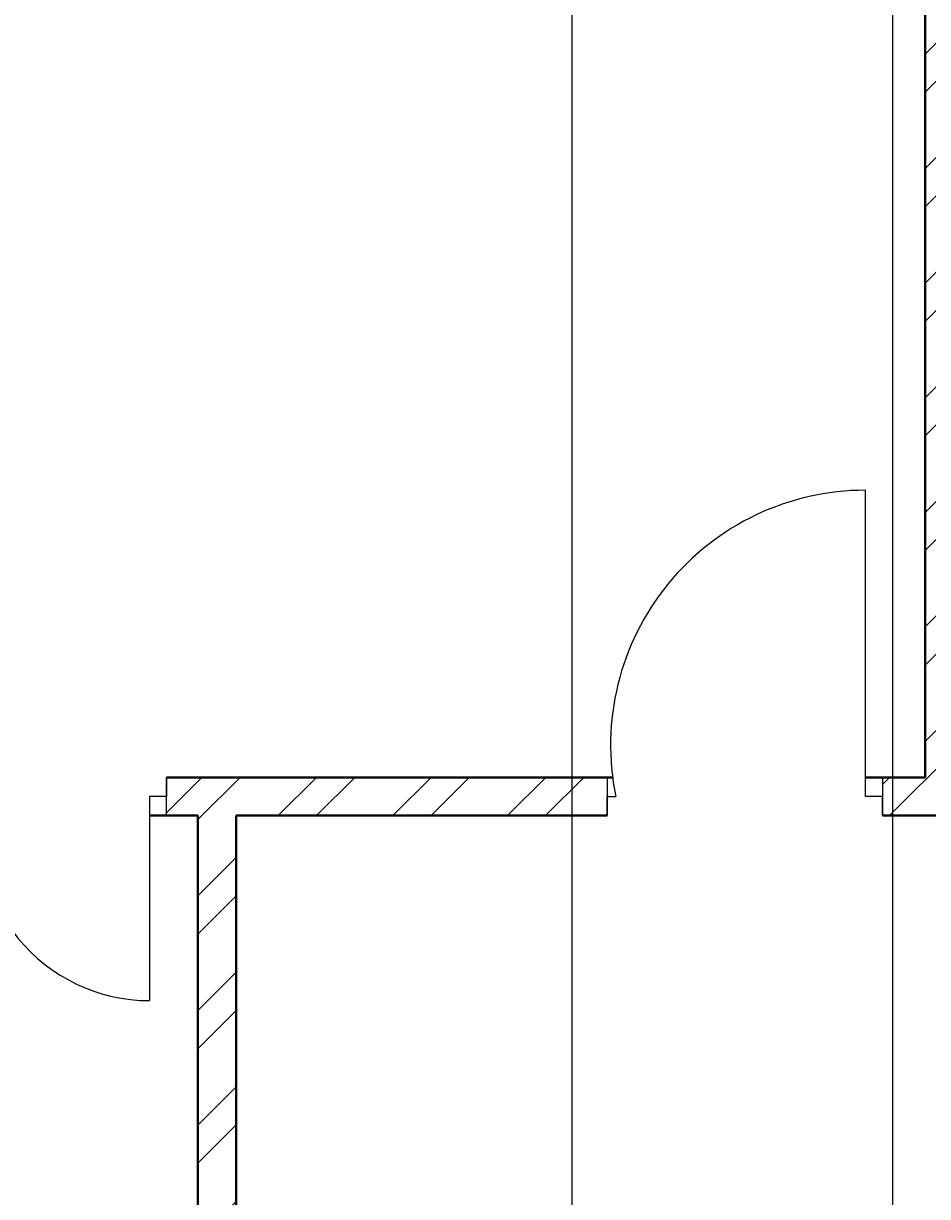
# Model space of a CAD drawing. Units: inches. Extents: x 1601 to 2297, y 1496 to 2631.
# Tile 8 of 57: x 1783 to 1889, y 1835 to 1973. Entities that reach past the tile are written whole.
import ezdxf

# ---------------------------------------------------------------- set-up
doc = ezdxf.new("R2010")
doc.units = ezdxf.units.IN
for name, color, linetype, lineweight in [('A-ANNO-DIMS', 2, 'Continuous', 18), ('A-DOOR', 21, 'Continuous', 25), ('A-WALL', 7, 'Continuous', 40), ('A-WALL-PATT', 215, 'Continuous', 13)]:
    doc.layers.add(name, color=color, linetype=linetype, lineweight=lineweight)
doc.styles.get("Standard").update_dxf_attribs({"font": 'arial.ttf'})
doc.dimstyles.get("Standard").update_dxf_attribs({"dimtxt": 0.18, "dimasz": 0.18, "dimexe": 0.18, "dimexo": 0.0625, "dimgap": 0.09, "dimtad": 0, "dimtih": 1, "dimtoh": 1, "dimdec": 4, "dimzin": 0, "dimdsep": 46, "dimtxsty": 'Standard', "dimcen": 0.09, "dimadec": 0, "dimazin": 0, "dimtfac": 1, "dimtdec": 4, "dimtofl": 0, "dimtmove": 0, "dimatfit": 3, "dimfxl": 1, "dimtolj": 1, "dimtzin": 0, "dimarcsym": 0})

# ---------------------------------------------------------------- blocks, each defined once
blk = doc.blocks.new('*D46')
at = {"layer": 'A-ANNO-DIMS', "color": 0, "lineweight": -2, "transparency": 16777216}
for p, q in [((1846.99, 2347.76), (1846.99, 1513.75)), ((1884.68, 2347.76), (1884.68, 1513.75)), ((1847.17, 1513.93), (1865.44, 1513.93)), ((1884.5, 1513.93), (1866.23, 1513.93))]:
    blk.add_line(p, q, dxfattribs=at)
at = {"layer": 'A-ANNO-DIMS', "color": 0, "transparency": 16777216}
for points in [[(1847.17, 1513.96), (1847.17, 1513.9), (1846.99, 1513.93)], [(1884.5, 1513.96), (1884.5, 1513.9), (1884.68, 1513.93)]]:
    blk.add_solid(points, dxfattribs=at)
at = {"layer": 'Defpoints', "color": 0, "transparency": 16777216}
for p in [(1846.99, 2347.83), (1884.68, 2347.83), (1884.68, 1513.93)]:
    blk.add_point(p, dxfattribs=at)
at = {"layer": 'A-ANNO-DIMS', "color": 0, "transparency": 16777216, "insert": (1865.84, 1513.93), "char_height": 0.18, "attachment_point": 5}
blk.add_mtext('\\A1;37.68', dxfattribs=at)

msp = doc.modelspace()

# ---------------------------------------------------------------- hatches: boundary and pattern name
at = {"layer": 'A-WALL-PATT'}
h = msp.add_hatch(dxfattribs=at)
h.set_pattern_fill('ANSI32', color=256)
h.paths.add_polyline_path([(2230.5373, 1861.8254), (2182.5373, 1861.8254), (2182.5373, 1885.3637), (2178.0373, 1885.3637), (2178.0373, 1861.8254), (2166.0373, 1861.8254), (2134.5373, 1861.8254), (2130.0373, 1861.8254), (2130.0373, 1841.4682), (2126.8833, 1841.4682), (2126.8833, 1836.9682), (2130.0373, 1836.9682), (2130.0373, 1822.7302), (2134.5373, 1822.7302), (2134.5373, 1857.3254), (2166.0373, 1857.3254), (2226.0373, 1857.3254), (2226.0373, 1846.1155), (2230.5373, 1846.1155)])
h.paths.add_polyline_path([(2226.0373, 1797.3254), (2134.5373, 1797.3254), (2134.5373, 1800.6636), (2132.2873, 1800.6636), (2130.0373, 1800.6636), (2130.0373, 1797.3254), (2130.0373, 1792.8254), (2167.7264, 1792.8254), (2226.0373, 1792.8254)])
h.paths.add_polyline_path([(2230.5373, 1822.1155), (2226.0373, 1822.1155), (2226.0373, 1760.8563), (2230.5373, 1760.8563)])
h.paths.add_polyline_path([(2230.5373, 1700.8563), (2226.0373, 1700.8563), (2226.0373, 1644.3254), (2140.2517, 1644.3254), (2140.2517, 1635.3254), (2230.5373, 1635.3254)])
h.paths.add_polyline_path([(2080.2517, 1639.8254), (2080.2517, 1644.3254), (2035.5373, 1644.3254), (2035.5373, 1792.8254), (2094.0373, 1792.8254), (2094.0373, 1797.3254), (2094.0373, 1836.9682), (2097.1057, 1836.9682), (2097.1057, 1839.2182), (2097.1057, 1841.4682), (2094.0373, 1841.4682), (2094.0373, 1862.2276), (2089.5373, 1862.2276), (2089.5373, 1797.3254), (2035.5373, 1797.3254), (2035.5373, 1857.3254), (2035.5373, 1885.0916), (2031.0373, 1885.0916), (2031.0373, 1710.3254), (2012.329, 1710.3254), (2012.329, 1701.3254), (2031.0373, 1701.3254), (2031.0373, 1644.3254), (2031.0373, 1635.3254), (2080.2517, 1635.3254)])
h.paths.add_polyline_path([(1836.0373, 1653.2033), (1842.6171, 1653.2033), (1842.6171, 1657.7033), (1842.6171, 1662.2033), (1831.5373, 1662.2033), (1831.5373, 1764.2033), (1835.3881, 1764.2033), (1835.3881, 1766.4533), (1835.3881, 1768.7033), (1831.5373, 1768.7033), (1827.0373, 1768.7033), (1827.0373, 1662.2033), (1827.0373, 1635.3254), (1836.0373, 1635.3254)])
h.paths.add_polyline_path([(1893.0373, 1701.3254), (1907.193, 1701.3254), (1907.193, 1705.8254), (1907.193, 1710.3254), (1893.0373, 1710.3254), (1893.0373, 1819.8254), (1882.6444, 1819.8254), (1882.6444, 1817.5754), (1882.6444, 1815.3254), (1888.5373, 1815.3254), (1888.5373, 1662.2033), (1884.0373, 1662.2033), (1866.6171, 1662.2033), (1866.6171, 1653.2033), (1882.391, 1653.2033), (1884.0373, 1653.2033), (1884.0373, 1635.3254), (1893.0373, 1635.3254)])
h.paths.add_polyline_path([(1739.3335, 1639.8254), (1739.3335, 1644.3254), (1695.0373, 1644.3254), (1695.0373, 1702.0135), (1690.5373, 1702.0135), (1686.0373, 1702.0135), (1686.0373, 1635.3254), (1739.3335, 1635.3254)])
h.paths.add_polyline_path([(1827.0373, 1644.3254), (1799.3335, 1644.3254), (1799.3335, 1635.3254), (1827.0373, 1635.3254)])
h.paths.add_polyline_path([(1695.0373, 1815.3254), (1849.2759, 1815.3254), (1849.2759, 1819.8254), (1807.5373, 1819.8254), (1807.5373, 1879.8254), (1851.1533, 1879.8254), (1851.1533, 1882.0754), (1851.1533, 1884.3254), (1799.3405, 1884.3254), (1799.3405, 1882.0754), (1799.3405, 1879.8254), (1803.0373, 1879.8254), (1803.0373, 1819.8254), (1695.0373, 1819.8254), (1695.0373, 1835.0458), (1690.5373, 1835.0458), (1686.0373, 1835.0458), (1686.0373, 1766.1753), (1695.0373, 1766.1753)])
h.paths.add_polyline_path([(1775.8157, 1884.3254), (1695.0373, 1884.3254), (1695.0373, 1912.9526), (1690.5373, 1912.9526), (1686.0373, 1912.9526), (1686.0373, 1859.0458), (1695.0373, 1859.0458), (1695.0373, 1879.8254), (1775.8157, 1879.8254)])
h.paths.add_polyline_path([(1893.0373, 2031.3254), (1731.5687, 2031.3254), (1731.5687, 2057.4352), (1722.5687, 2057.4352), (1722.5687, 2031.3254), (1686.0373, 2031.3254), (1686.0373, 1972.9526), (1695.0373, 1972.9526), (1695.0373, 2022.3254), (1888.5373, 2022.3254), (1888.5373, 1884.3254), (1883.4996, 1884.3254), (1883.4996, 1879.8254), (1893.0373, 1879.8254), (1893.0373, 1974.3254), (1976.6199, 1974.3254), (1976.6199, 1978.8254), (1968.0373, 1978.8254), (1968.0373, 1983.3254), (1968.0373, 2008.4756), (1963.5373, 2008.4756), (1959.0373, 2008.4756), (1959.0373, 1983.3254), (1893.0373, 1983.3254)])
h.paths.add_polyline_path([(2230.5373, 2140.4745), (2226.0373, 2140.4745), (2226.0373, 2094.3254), (2040.0373, 2094.3254), (2040.0373, 2085.3254), (2178.0373, 2085.3254), (2178.0373, 2065.6965), (2182.5373, 2065.6965), (2182.5373, 2085.3254), (2226.0373, 2085.3254), (2226.0373, 1986.3254), (2211.2679, 1986.3254), (2211.2679, 1981.8254), (2230.5373, 1981.8254)])
h.paths.add_polyline_path([(2187.6292, 1986.3254), (2182.5373, 1986.3254), (2182.5373, 2029.6965), (2178.0373, 2029.6965), (2178.0373, 1986.3254), (2099.05, 1986.3254), (2099.05, 1981.8254), (2178.0373, 1981.8254), (2178.0373, 1969.3637), (2182.5373, 1969.3637), (2182.5373, 1981.8254), (2187.6292, 1981.8254), (2187.6292, 1984.0754)])
h.paths.add_polyline_path([(1807.1169, 1573.5395), (2055.0405, 1573.5395), (2055.0405, 1610.6322), (1807.1169, 1610.6322)], flags=9)
h.paths.add_polyline_path([(1841.1631, 1712.7967), (1870.3957, 1712.7967), (1870.3957, 1731.454), (1841.1631, 1731.454)], flags=9)
h.paths.add_polyline_path([(2144.3862, 1772.185), (2191.0233, 1772.185), (2191.0233, 1790.8423), (2144.3862, 1790.8423)], flags=9)
h.paths.add_polyline_path([(2143.0128, 1827.3312), (2177.9958, 1827.3312), (2177.9958, 1845.9886), (2143.0128, 1845.9886)], flags=25)
h.paths.add_polyline_path([(2041.2439, 1833.5691), (2070.8516, 1833.5691), (2070.8516, 1852.2264), (2041.2439, 1852.2264)], flags=25)
h.paths.add_polyline_path([(2097.2791, 1947.0598), (2134.2061, 1947.0598), (2134.2061, 1965.7171), (2097.2791, 1965.7171)], flags=9)
h.paths.add_polyline_path([(2214.995, 1904.3124), (2214.995, 1942.2899), (2196.3376, 1942.2899), (2196.3376, 1904.3124)], flags=9)
h.paths.add_polyline_path([(2186.6284, 2043.8031), (2219.7935, 2043.8031), (2219.7935, 2062.4605), (2186.6284, 2062.4605)], flags=25)
h.paths.add_polyline_path([(2064.0877, 2031.616), (2097.4949, 2031.616), (2097.4949, 2050.2734), (2064.0877, 2050.2734)], flags=25)
h.paths.add_polyline_path([(1973.1349, 1986.0688), (2008.4009, 1986.0688), (2008.4009, 2004.7261), (1973.1349, 2004.7261)], flags=9)
h.paths.add_polyline_path([(1976.3676, 2106.9635), (2005.7469, 2106.9635), (2005.7469, 2125.6209), (1976.3676, 2125.6209)], flags=9)
h.paths.add_polyline_path([(1991.7852, 2180.4863), (2027.0513, 2180.4863), (2027.0513, 2199.1437), (1991.7852, 2199.1437)], flags=9)
h.paths.add_polyline_path([(2106.1801, 2187.9359), (2152.2101, 2187.9359), (2152.2101, 2206.5932), (2106.1801, 2206.5932)], flags=9)
h.paths.add_polyline_path([(2148.6686, 2262.2542), (2182.318, 2262.2542), (2182.318, 2280.9115), (2148.6686, 2280.9115)], flags=9)
h.paths.add_polyline_path([(2041.6327, 2252.8147), (2071.2405, 2252.8147), (2071.2405, 2271.4721), (2041.6327, 2271.4721)], flags=9)
h.paths.add_polyline_path([(2063.9734, 2375.4265), (2100.9004, 2375.4265), (2100.9004, 2394.0839), (2063.9734, 2394.0839)], flags=9)
h.paths.add_polyline_path([(2216.4955, 2330.9748), (2216.4955, 2370.2654), (2197.8381, 2370.2654), (2197.8381, 2330.9748)], flags=9)
h.paths.add_polyline_path([(2179.1416, 2485.8687), (2212.3067, 2485.8687), (2212.3067, 2504.5261), (2179.1416, 2504.5261)], flags=9)
h.paths.add_polyline_path([(2078.7442, 2471.1516), (2112.1514, 2471.1516), (2112.1514, 2489.809), (2078.7442, 2489.809)], flags=9)
h.paths.add_polyline_path([(1915.9631, 2329.4668), (1952.8902, 2329.4668), (1952.8902, 2348.1241), (1915.9631, 2348.1241)], flags=9)
h.paths.add_polyline_path([(1904.3189, 2499.6709), (1940.4512, 2499.6709), (1940.4512, 2518.3282), (1904.3189, 2518.3282)], flags=9)
h.paths.add_polyline_path([(1892.3665, 2100.4595), (1925.6374, 2100.4595), (1925.6374, 2119.1169), (1892.3665, 2119.1169)], flags=9)
h.paths.add_polyline_path([(1909.2984, 1805.9631), (1946.2254, 1805.9631), (1946.2254, 1824.6205), (1909.2984, 1824.6205)], flags=9)
h.paths.add_polyline_path([(1934.6056, 1658.616), (1970.738, 1658.616), (1970.738, 1677.2733), (1934.6056, 1677.2733)], flags=9)
h.paths.add_polyline_path([(1711.2052, 1789.8902), (1750.0456, 1789.8902), (1750.0456, 1808.5476), (1711.2052, 1808.5476)], flags=25)
h.paths.add_polyline_path([(1742.7874, 1854.6743), (1771.9449, 1854.6743), (1771.9449, 1873.3317), (1742.7874, 1873.3317)], flags=25)
h.paths.add_polyline_path([(1807.3592, 1997.7912), (1850.1116, 1997.7912), (1850.1116, 2016.4486), (1807.3592, 2016.4486)], flags=25)
h.paths.add_polyline_path([(1717.4579, 2237.7844), (1760.2103, 2237.7844), (1760.2103, 2256.4417), (1717.4579, 2256.4417)], flags=9)
h.paths.add_polyline_path([(1780.9285, 2324.0623), (1810.086, 2324.0623), (1810.086, 2342.7197), (1780.9285, 2342.7197)], flags=9)
h.paths.add_polyline_path([(1837.696, 2449.2024), (1866.9286, 2449.2024), (1866.9286, 2467.8598), (1837.696, 2467.8598)], flags=9)
h.paths.add_polyline_path([(1712.7752, 2484.9404), (1751.6156, 2484.9404), (1751.6156, 2503.5977), (1712.7752, 2503.5977)], flags=9)

# ---------------------------------------------------------------- linework, layer by layer
at = {"layer": 'A-DOOR'}
for p, q in [((1881.4996, 1882.0754), (1881.4996, 1918.0754)), ((1799.3405, 1879.8254), (1799.3405, 1884.3254)), ((1799.3405, 1884.3254), (1799.3405, 1882.0754)), ((1851.1533, 1884.3254), (1851.1533, 1879.8254)), ((1883.4996, 1884.3254), (1883.4996, 1879.8254)), ((1799.3405, 1882.0754), (1797.3405, 1882.0754)), ((1797.3405, 1882.0754), (1797.3405, 1858.0754)), ((1851.1533, 1879.8254), (1851.1533, 1882.0754)), ((1851.1533, 1882.0754), (1852.1533, 1882.0754)), ((1883.4996, 1882.0754), (1881.4996, 1882.0754)), ((1883.4996, 1879.8254), (1883.4996, 1882.0754))]:
    msp.add_line(p, q, dxfattribs=at)
for centre, radius, start, end in [((1881.4996, 1888.1142), 29.9612, 90, 191.627799), ((1797.3405, 1878.0174), 19.942, 168.258947, 270)]:
    msp.add_arc(centre, radius, start, end, dxfattribs=at)
at = {"layer": 'A-WALL'}
for p, q in [((1888.5373, 2022.3254), (1888.5373, 1884.3254)), ((1799.3405, 1884.3254), (1851.7789, 1884.3254)), ((1881.4996, 1884.3254), (1888.5373, 1884.3254)), ((1797.3405, 1879.8254), (1803.0373, 1879.8254)), ((1797.3405, 1879.8254), (1803.0373, 1879.8254)), ((1803.0373, 1879.8254), (1803.0373, 1819.8254)), ((1807.5373, 1819.8254), (1807.5373, 1879.8254)), ((1807.5373, 1879.8254), (1851.1533, 1879.8254)), ((1883.4996, 1879.8254), (1893.0373, 1879.8254))]:
    msp.add_line(p, q, dxfattribs=at)

# ---------------------------------------------------------------- dimensions: what is measured, and where the dimension line sits
at = {"layer": 'A-ANNO-DIMS'}
dim = msp.add_linear_dim(base=(1884.6773, 1513.9279), p1=(1846.9946, 2347.8254), p2=(1884.6773, 2347.8254), dimstyle='Standard', override={"dimdec": 2, "dimlfac": 1, "dimrnd": 0, "dimzin": 0, "dimdsep": 46, "dimlunit": 2}, dxfattribs=at)
dim.commit()
dim.dimension.update_dxf_attribs({"geometry": '*D46', "text_midpoint": (1865.836, 1513.9279)})

doc.saveas('drawing.dxf')
